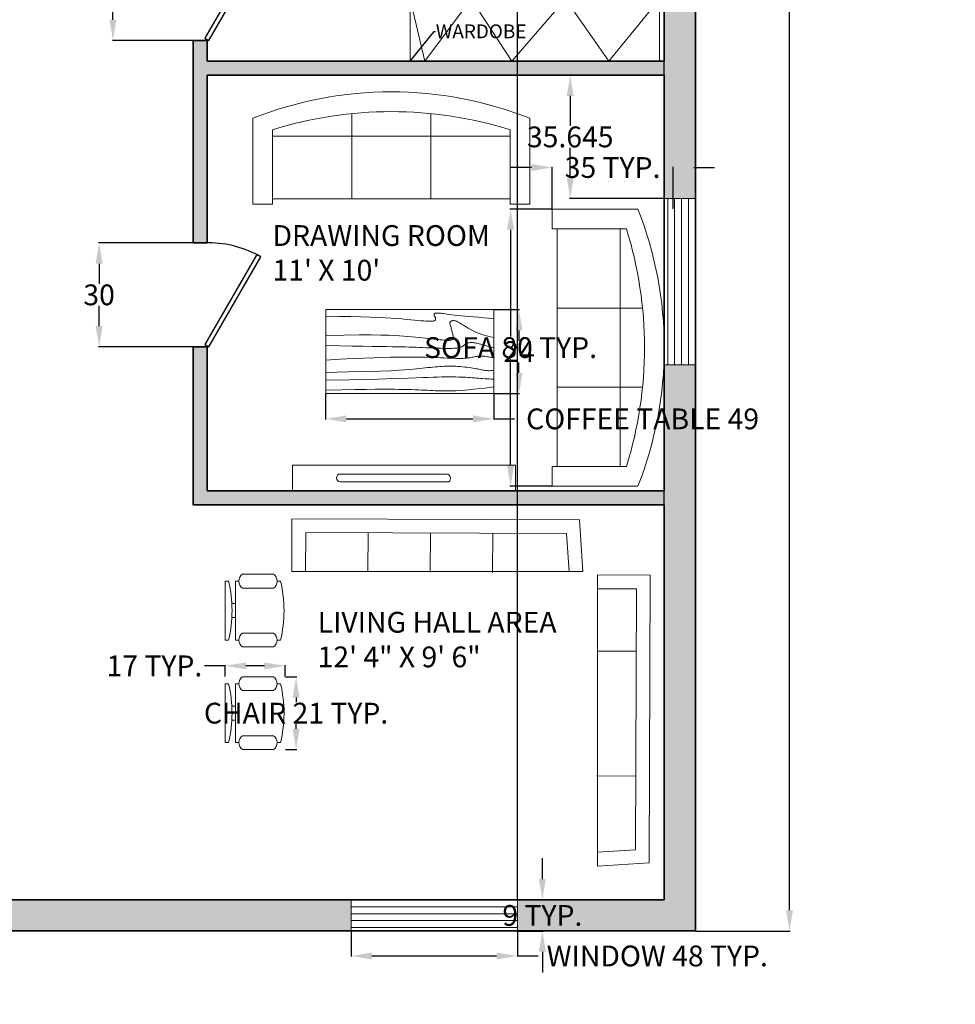
# Model space of a CAD drawing. Units: inches. Extents: x -16 to 578, y -553 to 49.
# Tile 2 of 5: x 308 to 578, y -543 to -259. Entities that reach past the tile are written whole.
import ezdxf
from ezdxf import colors
from ezdxf.entities.mleader import LeaderData, LeaderLine
from ezdxf.math import Vec2, Vec3

# ---------------------------------------------------------------- set-up
doc = ezdxf.new("R2010")
doc.units = ezdxf.units.IN
doc.header["$MEASUREMENT"] = 0
for name, color, linetype, lineweight in [('A-ANNO-DIMS', 2, 'Continuous', 18), ('A-ANNO-TEXT', 7, 'Continuous', 18), ('A-AREA-IDEN', 7, 'Continuous', 25), ('A-DOOR', 3, 'Continuous', 25), ('A-FLOR-CASE', 8, 'Continuous', 18), ('A-FURN', 8, 'Continuous', 18), ('A-GLAZ', 4, 'Continuous', 18), ('A-WALL', 7, 'Continuous', 35)]:
    doc.layers.add(name, color=color, linetype=linetype, lineweight=lineweight)
doc.layers.add('A-WALL-PATT', color=251, linetype='Continuous', lineweight=13, true_color=0x636466)
doc.styles.get("Standard").update_dxf_attribs({"font": 'arial.ttf'})
doc.dimstyles.get("Standard").update_dxf_attribs({"dimtxt": 6, "dimasz": 6, "dimexe": 0.18, "dimexo": 0.0625, "dimgap": 0.09, "dimtad": 0, "dimtih": 1, "dimtoh": 1, "dimdec": 0, "dimzin": 0, "dimdsep": 46, "dimlunit": 4, "dimtxsty": 'Standard', "dimcen": 0.09, "dimadec": 0, "dimazin": 0, "dimtfac": 1, "dimtdec": 0, "dimtofl": 0, "dimtmove": 0, "dimatfit": 3, "dimfxl": 1, "dimtolj": 1, "dimtzin": 0, "dimarcsym": 0})

# ---------------------------------------------------------------- blocks, each defined once
blk = doc.blocks.new('*U4')
for p, q in [((0, 0), (0, -6)), ((-40, 0), (-40, -6))]:
    blk.add_line(p, q)
blk.add_lwpolyline([(0, 0), (-34.64, 20), (-35.52, 18.48), (-0.88, -1.52)], close=True)
blk.add_arc((0, 0), 40, 150, 180)
blk = doc.blocks.new('Chair - Desk')
for p, q in [((-8.5, 0), (-8.5, -1)), ((-8.5, 0), (8.5, 0)), ((8.5, 0), (8.5, -1)), ((-2, -3), (-2, -1.9355)), ((2, -1.9576), (2, -3)), ((-10.5, -5), (-10.5, -14)), ((-8.5, -3), (-8.5, -4)), ((-8.5, -3), (8.5, -3)), ((-6.5, -14), (-6.5, -5)), ((6.5, -5), (6.5, -14)), ((8.5, -3), (8.5, -4)), ((10.5, -14), (10.5, -5)), ((-8.5, -15), (-8.5, -16)), ((8.5, -15), (8.5, -16))]:
    blk.add_line(p, q)
for centre, radius, start, end in [((0, 34.625), 36.625, 256.5803, 283.4197), ((-8.5, -6.5), 2.5, 36.8699, 143.1301), ((8.5, -6.5), 2.5, 36.8699, 143.1301), ((-8.5, -12.5), 2.5, 216.8699, 323.1301), ((8.5, -12.5), 2.5, 216.8699, 323.1301), ((0, 19.625), 36.625, 256.5803, 283.4197)]:
    blk.add_arc(centre, radius, start, end)
blk = doc.blocks.new('Table - Rectangular Woodgrain 60 x 30 in.')
for p, q in [((0, 0), (0, -30)), ((60, 0), (0, 0)), ((60, -30), (60, 0)), ((0, -30), (60, -30))]:
    blk.add_line(p, q)
for points in [[(0, -2.4), (4.8155, -2.418), (9.0302, -2.4688), (12.709, -2.5477), (15.9167, -2.65), (18.7181, -2.7711), (21.1781, -2.9063), (23.3616, -3.0508), (25.3333, -3.2), (27.1477, -3.3495), (28.8172, -3.4958), (30.3437, -3.636), (31.7291, -3.7667), (32.9756, -3.8849), (34.0849, -3.9875), (35.059, -4.0714), (35.9, -4.1334), (36.6114, -4.1711), (37.2041, -4.1854), (37.6906, -4.1779), (38.0833, -4.15), (38.3948, -4.1034), (38.6375, -4.0396), (38.8239, -3.9602), (38.9666, -3.8667), (39.0764, -3.7608), (39.1573, -3.6448), (39.2116, -3.521), (39.2416, -3.3917), (39.2498, -3.2593), (39.2385, -3.1261), (39.21, -2.9944), (39.1666, -2.8667), (39.111, -2.7447), (39.0468, -2.6281), (38.978, -2.5163), (38.9083, -2.4083), (38.8418, -2.3035), (38.7823, -2.201), (38.7337, -2.1001), (38.7, -2), (38.6844, -1.9003), (38.6875, -1.8021), (38.7094, -1.707), (38.75, -1.6167), (38.8094, -1.5326), (38.8875, -1.4563), (38.9844, -1.3893), (39.1, -1.3333), (39.2351, -1.2896), (39.3937, -1.2583), (39.5804, -1.2396), (39.8, -1.2333), (40.057, -1.2396), (40.3562, -1.2583), (40.7023, -1.2896), (41.1, -1.3333), (41.5547, -1.3895), (42.0755, -1.4573), (42.6721, -1.5361), (43.3542, -1.625), (44.1316, -1.7233), (45.014, -1.8302), (46.0114, -1.9449), (47.1333, -2.0667), (48.3862, -2.1947), (49.7625, -2.3281), (51.2513, -2.4663), (52.8416, -2.6083), (54.5226, -2.7535), (56.2833, -2.9011), (58.1127, -3.0501), (60, -3.2)], [(0, -9.2), (6.5759, -9.0858), (11.9385, -9.0365), (16.2527, -9.0418), (19.6833, -9.0917), (22.3952, -9.1759), (24.5531, -9.2844), (26.322, -9.4069), (27.8666, -9.5333), (29.3241, -9.6553), (30.7203, -9.7719), (32.0532, -9.8837), (33.3208, -9.9917), (34.5213, -10.0965), (35.6526, -10.199), (36.7128, -10.2999), (37.7, -10.4), (38.6129, -10.4996), (39.4531, -10.5969), (40.223, -10.6895), (40.925, -10.775), (41.5613, -10.8512), (42.1344, -10.9156), (42.6465, -10.966), (43.1, -11), (43.4976, -11.0158), (43.8437, -11.0136), (44.143, -10.9942), (44.4, -10.9583), (44.6195, -10.9069), (44.8062, -10.8406), (44.9648, -10.7603), (45.1, -10.6667), (45.2155, -10.5598), (45.3114, -10.4365), (45.3871, -10.2929), (45.4416, -10.125), (45.4743, -9.929), (45.4844, -9.7011), (45.4709, -9.4371), (45.4333, -9.1333), (45.3716, -8.7883), (45.2896, -8.4104), (45.1919, -8.0107), (45.0833, -7.6), (44.9685, -7.1893), (44.8521, -6.7896), (44.7388, -6.4117), (44.6333, -6.0667), (44.54, -5.7628), (44.4614, -5.4979), (44.4001, -5.2675), (44.3583, -5.0667), (44.3384, -4.8909), (44.3427, -4.7354), (44.3736, -4.5956), (44.4333, -4.4667), (44.5236, -4.3453), (44.6427, -4.2333), (44.7884, -4.1339), (44.9583, -4.05), (45.1501, -3.9849), (45.3614, -3.9417), (45.59, -3.9234), (45.8333, -3.9333), (46.0915, -3.9749), (46.3734, -4.0531), (46.6906, -4.1736), (47.0542, -4.3417), (47.4756, -4.5629), (47.9661, -4.8427), (48.5372, -5.1866), (49.2, -5.6), (49.9676, -6.0844), (50.8594, -6.625), (51.8965, -7.2031), (53.1, -7.8), (54.491, -8.3969), (56.0906, -8.975), (57.9199, -9.5156), (60, -10)], [(0, -12.8), (5.1847, -12.9322), (9.6213, -13.0323), (13.3963, -13.1059), (16.5958, -13.1583), (19.3063, -13.1952), (21.614, -13.2219), (23.6054, -13.2439), (25.3666, -13.2667), (26.9728, -13.2947), (28.4531, -13.3281), (29.8256, -13.3663), (31.1083, -13.4083), (32.3191, -13.4535), (33.476, -13.501), (34.597, -13.5501), (35.7, -13.6), (36.7984, -13.6497), (37.8875, -13.6979), (38.9578, -13.743), (40, -13.7833), (41.0047, -13.8174), (41.9625, -13.8438), (42.864, -13.8607), (43.7, -13.8667), (44.4631, -13.8604), (45.1552, -13.8417), (45.7801, -13.8104), (46.3416, -13.7667), (46.8439, -13.7104), (47.2906, -13.6417), (47.6858, -13.5604), (48.0333, -13.4667), (48.3375, -13.3608), (48.6042, -13.2448), (48.8396, -13.121), (49.05, -12.9917), (49.2417, -12.8593), (49.4208, -12.7261), (49.5937, -12.5944), (49.7667, -12.4667), (49.9452, -12.3451), (50.1323, -12.2313), (50.3303, -12.1268), (50.5416, -12.0333), (50.7686, -11.9524), (51.0135, -11.8854), (51.2788, -11.8341), (51.5666, -11.8), (51.8785, -11.7843), (52.2116, -11.7865), (52.562, -11.8059), (52.926, -11.8417), (53.2998, -11.8931), (53.6795, -11.9594), (54.0614, -12.0397), (54.4416, -12.1333), (54.8223, -12.2401), (55.2293, -12.3625), (55.6942, -12.5037), (56.2489, -12.6667), (56.9251, -12.8547), (57.7545, -13.0708), (58.7689, -13.3182), (60, -13.6)], [(0, -18), (5.124, -17.7273), (9.6609, -17.5057), (13.6705, -17.3303), (17.2125, -17.1958), (20.3467, -17.0973), (23.1328, -17.0297), (25.6307, -16.9878), (27.9, -16.9667), (29.9928, -16.9617), (31.9302, -16.9703), (33.7254, -16.9907), (35.3917, -17.0208), (36.9423, -17.0588), (38.3906, -17.1026), (39.7499, -17.1503), (41.0333, -17.2), (42.2519, -17.2496), (43.4073, -17.2969), (44.4986, -17.3395), (45.525, -17.375), (46.4858, -17.4012), (47.3802, -17.4156), (48.2074, -17.416), (48.9667, -17.4), (49.6583, -17.3662), (50.2872, -17.3167), (50.8595, -17.2547), (51.3812, -17.1833), (51.8584, -17.1057), (52.2971, -17.025), (52.7034, -16.9443), (53.0833, -16.8667), (53.443, -16.7951), (53.789, -16.7313), (54.128, -16.6768), (54.4666, -16.6334), (54.8115, -16.6024), (55.1693, -16.5854), (55.5465, -16.5841), (55.95, -16.6), (56.3828, -16.6337), (56.8346, -16.6823), (57.2915, -16.7418), (57.7396, -16.8084), (58.165, -16.878), (58.5539, -16.9469), (58.8924, -17.0111), (59.1666, -17.0667), (59.3679, -17.1107), (59.5078, -17.1438), (59.6032, -17.1675), (59.6708, -17.1833), (59.7275, -17.193), (59.7901, -17.1979), (59.8753, -17.1998), (60, -17.2)], [(0, -22.4), (8.0098, -22.2501), (14.4094, -22.1011), (19.4168, -21.9535), (23.25, -21.8083), (26.1269, -21.6663), (28.2656, -21.5281), (29.884, -21.3947), (31.2, -21.2667), (32.3967, -21.1448), (33.5172, -21.0292), (34.5697, -20.9198), (35.5625, -20.8167), (36.5037, -20.7198), (37.4015, -20.6292), (38.2642, -20.5448), (39.1, -20.4667), (39.9164, -20.3951), (40.7187, -20.3313), (41.5117, -20.2768), (42.3, -20.2333), (43.0883, -20.2024), (43.8812, -20.1854), (44.6836, -20.1841), (45.5, -20.2), (46.3328, -20.234), (47.1747, -20.2844), (48.0163, -20.3488), (48.8479, -20.425), (49.66, -20.5106), (50.4429, -20.6031), (51.1872, -20.7004), (51.8833, -20.8), (52.5246, -20.8999), (53.1166, -20.9995), (53.6681, -21.0983), (54.1875, -21.1958), (54.6834, -21.2919), (55.1646, -21.3859), (55.6394, -21.4777), (56.1167, -21.5667), (56.6028, -21.6515), (57.0961, -21.7266), (57.5929, -21.7852), (58.0896, -21.8208), (58.5823, -21.8268), (59.0674, -21.7964), (59.5412, -21.723), (60, -21.6)], [(0, -25.2), (8.6355, -25.0504), (15.7026, -24.9031), (21.4049, -24.7606), (25.9458, -24.625), (29.529, -24.4988), (32.3578, -24.3844), (34.6359, -24.284), (36.5667, -24.2), (38.3213, -24.1341), (39.9417, -24.0854), (41.437, -24.0523), (42.8167, -24.0333), (44.0901, -24.0268), (45.2667, -24.0313), (46.3557, -24.0451), (47.3667, -24.0667), (48.309, -24.0947), (49.1928, -24.1287), (50.0284, -24.168), (50.826, -24.2125), (51.5959, -24.2617), (52.3483, -24.3151), (53.0935, -24.3725), (53.8417, -24.4334), (54.6009, -24.497), (55.3699, -24.561), (56.1454, -24.6226), (56.9239, -24.6792), (57.7021, -24.7279), (58.4764, -24.7662), (59.2435, -24.7911), (60, -24.8)], [(0, -28.8), (5.6867, -28.6681), (10.45, -28.5698), (14.407, -28.5012), (17.675, -28.4584), (20.3711, -28.4374), (22.6125, -28.4344), (24.5164, -28.4455), (26.2, -28.4667), (27.762, -28.4947), (29.2276, -28.5281), (30.6033, -28.5663), (31.8958, -28.6084), (33.1118, -28.6535), (34.2578, -28.7011), (35.3405, -28.7501), (36.3666, -28.8), (37.3443, -28.8497), (38.288, -28.8974), (39.2137, -28.9412), (40.1375, -28.9792), (41.0753, -29.0093), (42.0432, -29.0297), (43.0572, -29.0384), (44.1333, -29.0333), (45.2936, -29.0114), (46.5843, -28.9641), (48.0579, -28.8816), (49.7666, -28.7542), (51.7629, -28.5721), (54.0989, -28.3255), (56.8272, -28.0048), (60, -27.6)]]:
    blk.add_lwpolyline(points)
blk = doc.blocks.new('Sofa - Roundback 7 ft.')
for p, q in [((-12.00002, -32.4421), (-12.00003, -6.5971)), ((11.99997, -32.4421), (11.99998, -6.5971)), ((-36.000027, -34), (-36.000027, -11.4696)), ((35.99998, -34), (35.99998, -11.4696)), ((-35.999844, -13.3819), (35.9998, -13.3819)), ((-36.000027, -32.4421), (35.99998, -32.4421))]:
    blk.add_line(p, q)
for points in [[(-36.000027, -34), (-42.000027, -34), (-42.000027, -8)], [(41.99998, -8), (41.99998, -34), (35.99998, -34)]]:
    blk.add_lwpolyline(points)
for centre, radius, start, end in [((0, -114.25), 114.25, 68.43141, 111.5686), ((-0.00001, -127.1968), 121.1968, 72.72033, 107.2797)]:
    blk.add_arc(centre, radius, start, end)
blk = doc.blocks.new('WIN-48X9')
for p, q in [((-48, -4), (0, -4)), ((-48, -6), (0, -6)), ((-48, -8), (0, -8))]:
    blk.add_line(p, q)
for points in [[(0, 0), (0, -9), (-48, -9), (-48, 0)], [(-48, -2), (0, -2)]]:
    blk.add_lwpolyline(points, close=True)
blk = doc.blocks.new('WARDROBE-72X18')
for p, q in [((0, 0), (18, -14.58)), ((18, -14.58), (0, -27.16)), ((0, -27.16), (18, -42.59)), ((18, -42.59), (0, -54.31)), ((0, -54.31), (18, -67.75)), ((18, -67.75), (0, -72))]:
    blk.add_line(p, q)
blk.add_lwpolyline([(0, 0), (18, 0), (18, -72), (0, -72)], close=True)
blk = doc.blocks.new('*D26')
at = {"layer": 'A-ANNO-DIMS', "color": 0, "lineweight": -2, "transparency": 16777216}
for p, q in [((403.8, -521.83), (403.8, -529.15)), ((451.8, -521.83), (451.8, -529.15)), ((409.8, -528.97), (445.8, -528.97)), ((451.8, -528.97), (457.8, -528.97))]:
    blk.add_line(p, q, dxfattribs=at)
at = {"layer": 'A-ANNO-DIMS', "color": 0, "transparency": 16777216}
for points in [[(409.8, -527.97), (409.8, -529.97), (403.8, -528.97)], [(445.8, -527.97), (445.8, -529.97), (451.8, -528.97)]]:
    blk.add_solid(points, dxfattribs=at)
at = {"layer": 'Defpoints', "color": 0, "transparency": 16777216}
for p in [(403.8, -521.77), (451.8, -521.77), (451.8, -528.97)]:
    blk.add_point(p, dxfattribs=at)
at = {"layer": 'A-ANNO-DIMS', "color": 0, "transparency": 16777216, "insert": (492.17, -528.97), "char_height": 6, "attachment_point": 5}
blk.add_mtext('\\A1;WINDOW 48 TYP.', dxfattribs=at)
blk = doc.blocks.new('*D27')
at = {"layer": 'A-ANNO-DIMS', "color": 0, "lineweight": -2, "transparency": 16777216}
for p, q in [((459, -506.77), (459, -500.77)), ((451.87, -512.77), (459.18, -512.77)), ((451.87, -521.77), (459.18, -521.77)), ((459, -527.77), (459, -533.77))]:
    blk.add_line(p, q, dxfattribs=at)
at = {"layer": 'A-ANNO-DIMS', "color": 0, "transparency": 16777216}
for points in [[(458, -506.77), (460, -506.77), (459, -512.77)], [(458, -527.77), (460, -527.77), (459, -521.77)]]:
    blk.add_solid(points, dxfattribs=at)
at = {"layer": 'Defpoints', "color": 0, "transparency": 16777216}
for p in [(451.8, -512.77), (459, -512.77), (451.8, -521.77)]:
    blk.add_point(p, dxfattribs=at)
at = {"layer": 'A-ANNO-DIMS', "color": 0, "transparency": 16777216, "insert": (459, -517.27), "char_height": 6, "attachment_point": 5}
blk.add_mtext('\\A1;9 TYP.', dxfattribs=at)
blk = doc.blocks.new('*D28')
at = {"layer": 'A-ANNO-DIMS', "color": 0, "lineweight": -2, "transparency": 16777216}
for p, q in [((471.56, -245.54), (471.56, -248.36)), ((489.56, -245.54), (489.56, -248.36)), ((477.56, -248.18), (483.56, -248.18)), ((489.56, -248.18), (495.56, -248.18))]:
    blk.add_line(p, q, dxfattribs=at)
at = {"layer": 'A-ANNO-DIMS', "color": 0, "transparency": 16777216}
for points in [[(477.56, -247.18), (477.56, -249.18), (471.56, -248.18)], [(483.56, -247.18), (483.56, -249.18), (489.56, -248.18)]]:
    blk.add_solid(points, dxfattribs=at)
at = {"layer": 'Defpoints', "color": 0, "transparency": 16777216}
for p in [(471.56, -245.48), (489.56, -245.48), (489.56, -248.18)]:
    blk.add_point(p, dxfattribs=at)
at = {"layer": 'A-ANNO-DIMS', "color": 0, "transparency": 16777216, "insert": (538.51, -248.18), "char_height": 6, "attachment_point": 5}
blk.add_mtext('\\A1;NIGHTSTAND 18 TYP.', dxfattribs=at)
blk = doc.blocks.new('*D36')
at = {"layer": 'A-ANNO-DIMS', "color": 0, "lineweight": -2, "transparency": 16777216}
for p, q in [((384.81, -448.4), (388.08, -448.4)), ((387.9, -454.4), (387.9, -455.71)), ((387.9, -463.4), (387.9, -462.09)), ((384.81, -469.4), (388.08, -469.4))]:
    blk.add_line(p, q, dxfattribs=at)
at = {"layer": 'A-ANNO-DIMS', "color": 0, "transparency": 16777216}
for points in [[(386.9, -454.4), (388.9, -454.4), (387.9, -448.4)], [(386.9, -463.4), (388.9, -463.4), (387.9, -469.4)]]:
    blk.add_solid(points, dxfattribs=at)
at = {"layer": 'Defpoints', "color": 0, "transparency": 16777216}
for p in [(384.75, -448.4), (387.9, -448.4), (384.75, -469.4)]:
    blk.add_point(p, dxfattribs=at)
at = {"layer": 'A-ANNO-DIMS', "color": 0, "transparency": 16777216, "insert": (387.9, -458.9), "char_height": 6, "attachment_point": 5}
blk.add_mtext('\\A1;CHAIR 21 TYP.', dxfattribs=at)
blk = doc.blocks.new('*D37')
at = {"layer": 'A-ANNO-DIMS', "color": 0, "lineweight": -2, "transparency": 16777216}
for p, q in [((367.42, -445.25), (361.42, -445.25)), ((367.42, -448.34), (367.42, -445.07)), ((378.75, -445.25), (373.42, -445.25)), ((384.75, -448.34), (384.75, -445.07))]:
    blk.add_line(p, q, dxfattribs=at)
at = {"layer": 'A-ANNO-DIMS', "color": 0, "transparency": 16777216}
for points in [[(373.42, -444.25), (373.42, -446.25), (367.42, -445.25)], [(378.75, -444.25), (378.75, -446.25), (384.75, -445.25)]]:
    blk.add_solid(points, dxfattribs=at)
at = {"layer": 'Defpoints', "color": 0, "transparency": 16777216}
for p in [(367.42, -445.25), (367.42, -448.4), (384.75, -448.4)]:
    blk.add_point(p, dxfattribs=at)
at = {"layer": 'A-ANNO-DIMS', "color": 0, "transparency": 16777216, "insert": (347.01, -445.25), "char_height": 6, "attachment_point": 5}
blk.add_mtext('\\A1;17 TYP.', dxfattribs=at)
blk = doc.blocks.new('*D42')
at = {"layer": 'A-ANNO-DIMS', "color": 0, "lineweight": -2, "transparency": 16777216}
for p, q in [((461.75, -313.41), (449.64, -313.41)), ((449.82, -319.41), (449.82, -350.21)), ((449.82, -387.39), (449.82, -356.6)), ((461.75, -393.39), (449.64, -393.39))]:
    blk.add_line(p, q, dxfattribs=at)
at = {"layer": 'A-ANNO-DIMS', "color": 0, "transparency": 16777216}
for points in [[(448.82, -319.41), (450.82, -319.41), (449.82, -313.41)], [(448.82, -387.39), (450.82, -387.39), (449.82, -393.39)]]:
    blk.add_solid(points, dxfattribs=at)
at = {"layer": 'Defpoints', "color": 0, "transparency": 16777216}
for p in [(449.82, -313.41), (461.82, -313.41), (461.82, -393.39)]:
    blk.add_point(p, dxfattribs=at)
at = {"layer": 'A-ANNO-DIMS', "color": 0, "transparency": 16777216, "insert": (449.82, -353.4), "char_height": 6, "attachment_point": 5}
blk.add_mtext('\\A1;SOFA 80 TYP.', dxfattribs=at)
blk = doc.blocks.new('*D43')
at = {"layer": 'A-ANNO-DIMS', "color": 0, "lineweight": -2, "transparency": 16777216}
for p, q in [((455.82, -301.42), (449.82, -301.42)), ((461.82, -313.35), (461.82, -301.24)), ((496.73, -313.35), (496.73, -301.24)), ((502.73, -301.42), (508.73, -301.42))]:
    blk.add_line(p, q, dxfattribs=at)
at = {"layer": 'A-ANNO-DIMS', "color": 0, "transparency": 16777216}
for points in [[(455.82, -300.42), (455.82, -302.42), (461.82, -301.42)], [(502.73, -300.42), (502.73, -302.42), (496.73, -301.42)]]:
    blk.add_solid(points, dxfattribs=at)
at = {"layer": 'Defpoints', "color": 0, "transparency": 16777216}
for p in [(496.73, -301.42), (461.82, -313.41), (496.73, -313.41)]:
    blk.add_point(p, dxfattribs=at)
at = {"layer": 'A-ANNO-DIMS', "color": 0, "transparency": 16777216, "insert": (479.27, -301.42), "char_height": 6, "attachment_point": 5}
blk.add_mtext('\\A1;35 TYP.', dxfattribs=at)
blk = doc.blocks.new('*D58')
at = {"layer": 'A-ANNO-DIMS', "color": 0, "lineweight": -2, "transparency": 16777216}
for p, q in [((396.44, -366.75), (396.44, -374.15)), ((444.97, -366.75), (444.97, -374.15)), ((402.44, -373.97), (438.97, -373.97)), ((444.97, -373.97), (450.97, -373.97))]:
    blk.add_line(p, q, dxfattribs=at)
at = {"layer": 'A-ANNO-DIMS', "color": 0, "transparency": 16777216}
for points in [[(402.44, -372.97), (402.44, -374.97), (396.44, -373.97)], [(438.97, -372.97), (438.97, -374.97), (444.97, -373.97)]]:
    blk.add_solid(points, dxfattribs=at)
at = {"layer": 'Defpoints', "color": 0, "transparency": 16777216}
for p in [(396.44, -366.69), (444.97, -366.69), (444.97, -373.97)]:
    blk.add_point(p, dxfattribs=at)
at = {"layer": 'A-ANNO-DIMS', "color": 0, "transparency": 16777216, "insert": (487.93, -373.97), "char_height": 6, "attachment_point": 5}
blk.add_mtext('\\A1;COFFEE TABLE 49', dxfattribs=at)
blk = doc.blocks.new('*D59')
at = {"layer": 'A-ANNO-DIMS', "color": 0, "lineweight": -2, "transparency": 16777216}
for p, q in [((445.03, -342.43), (452.43, -342.43)), ((452.25, -348.43), (452.25, -351.46)), ((452.25, -360.69), (452.25, -357.66)), ((445.03, -366.69), (452.43, -366.69))]:
    blk.add_line(p, q, dxfattribs=at)
at = {"layer": 'A-ANNO-DIMS', "color": 0, "transparency": 16777216}
for points in [[(451.25, -348.43), (453.25, -348.43), (452.25, -342.43)], [(451.25, -360.69), (453.25, -360.69), (452.25, -366.69)]]:
    blk.add_solid(points, dxfattribs=at)
at = {"layer": 'Defpoints', "color": 0, "transparency": 16777216}
for p in [(444.97, -342.43), (452.25, -342.43), (444.97, -366.69)]:
    blk.add_point(p, dxfattribs=at)
at = {"layer": 'A-ANNO-DIMS', "color": 0, "transparency": 16777216, "insert": (452.25, -354.56), "char_height": 6, "attachment_point": 5}
blk.add_mtext('\\A1;24', dxfattribs=at)
blk = doc.blocks.new('*D63')
at = {"layer": 'A-ANNO-DIMS', "color": 0, "lineweight": -2, "transparency": 16777216}
for p, q in [((503.25, 18.23), (530.52, 18.23)), ((530.34, 12.23), (530.34, -248.61)), ((530.34, -515.77), (530.34, -254.92)), ((503.25, -521.77), (530.52, -521.77))]:
    blk.add_line(p, q, dxfattribs=at)
at = {"layer": 'A-ANNO-DIMS', "color": 0, "transparency": 16777216}
for points in [[(529.34, 12.23), (531.34, 12.23), (530.34, 18.23)], [(529.34, -515.77), (531.34, -515.77), (530.34, -521.77)]]:
    blk.add_solid(points, dxfattribs=at)
at = {"layer": 'Defpoints', "color": 0, "transparency": 16777216}
for p in [(503.19, 18.23), (503.19, -521.77), (530.34, -521.77)]:
    blk.add_point(p, dxfattribs=at)
at = {"layer": 'A-ANNO-DIMS', "color": 0, "transparency": 16777216, "insert": (530.34, -251.77), "char_height": 6, "attachment_point": 5}
blk.add_mtext('\\A1;540', dxfattribs=at)
blk = doc.blocks.new('*D70')
at = {"layer": 'A-ANNO-DIMS', "color": 0, "lineweight": -2, "transparency": 16777216}
for p, q in [((362.13, -234.77), (334.86, -234.77)), ((335.04, -240.77), (335.04, -246.61)), ((335.04, -258.77), (335.04, -252.92)), ((362.13, -264.77), (334.86, -264.77))]:
    blk.add_line(p, q, dxfattribs=at)
at = {"layer": 'A-ANNO-DIMS', "color": 0, "transparency": 16777216}
for points in [[(334.04, -240.77), (336.04, -240.77), (335.04, -234.77)], [(334.04, -258.77), (336.04, -258.77), (335.04, -264.77)]]:
    blk.add_solid(points, dxfattribs=at)
at = {"layer": 'Defpoints', "color": 0, "transparency": 16777216}
for p in [(335.04, -234.77), (362.19, -234.77), (362.19, -264.77)]:
    blk.add_point(p, dxfattribs=at)
at = {"layer": 'A-ANNO-DIMS', "color": 0, "transparency": 16777216, "insert": (335.04, -249.77), "char_height": 6, "attachment_point": 5}
blk.add_mtext('\\A1;30', dxfattribs=at)
blk = doc.blocks.new('*D77')
at = {"layer": 'A-ANNO-DIMS', "color": 0, "lineweight": -2, "transparency": 16777216}
for p, q in [((494.13, -274.77), (466.86, -274.77)), ((467.04, -280.77), (467.04, -289.43)), ((467.04, -304.41), (467.04, -295.74)), ((494.13, -310.41), (466.86, -310.41))]:
    blk.add_line(p, q, dxfattribs=at)
at = {"layer": 'A-ANNO-DIMS', "color": 0, "transparency": 16777216}
for points in [[(466.04, -280.77), (468.04, -280.77), (467.04, -274.77)], [(466.04, -304.41), (468.04, -304.41), (467.04, -310.41)]]:
    blk.add_solid(points, dxfattribs=at)
at = {"layer": 'Defpoints', "color": 0, "transparency": 16777216}
for p in [(467.04, -274.77), (494.19, -274.77), (494.19, -310.41)]:
    blk.add_point(p, dxfattribs=at)
at = {"layer": 'A-ANNO-DIMS', "color": 0, "transparency": 16777216, "insert": (467.04, -292.59), "char_height": 6, "attachment_point": 5}
blk.add_mtext('\\A1;35.645', dxfattribs=at)
blk = doc.blocks.new('*D80')
at = {"layer": 'A-ANNO-DIMS', "color": 0, "lineweight": -2, "transparency": 16777216}
for p, q in [((451.8, -512.7), (451.8, 45.56)), ((494.19, -512.7), (494.19, 45.56)), ((457.8, 45.38), (462.66, 45.38)), ((488.19, 45.38), (483.34, 45.38))]:
    blk.add_line(p, q, dxfattribs=at)
at = {"layer": 'A-ANNO-DIMS', "color": 0, "transparency": 16777216}
for points in [[(457.8, 46.38), (457.8, 44.38), (451.8, 45.38)], [(488.19, 46.38), (488.19, 44.38), (494.19, 45.38)]]:
    blk.add_solid(points, dxfattribs=at)
at = {"layer": 'Defpoints', "color": 0, "transparency": 16777216}
for p in [(451.8, 45.38), (451.8, -512.77), (494.19, -512.77)]:
    blk.add_point(p, dxfattribs=at)
at = {"layer": 'A-ANNO-DIMS', "color": 0, "transparency": 16777216, "insert": (473, 45.38), "char_height": 6, "attachment_point": 5}
blk.add_mtext('\\A1;42.38', dxfattribs=at)
blk = doc.blocks.new('*D85')
at = {"layer": 'A-ANNO-DIMS', "color": 0, "lineweight": -2, "transparency": 16777216}
for p, q in [((358.13, -323.18), (330.86, -323.18)), ((331.04, -329.18), (331.04, -335.02)), ((331.04, -347.18), (331.04, -341.33)), ((358.13, -353.18), (330.86, -353.18))]:
    blk.add_line(p, q, dxfattribs=at)
at = {"layer": 'A-ANNO-DIMS', "color": 0, "transparency": 16777216}
for points in [[(330.04, -329.18), (332.04, -329.18), (331.04, -323.18)], [(330.04, -347.18), (332.04, -347.18), (331.04, -353.18)]]:
    blk.add_solid(points, dxfattribs=at)
at = {"layer": 'Defpoints', "color": 0, "transparency": 16777216}
for p in [(331.04, -323.18), (358.19, -323.18), (358.19, -353.18)]:
    blk.add_point(p, dxfattribs=at)
at = {"layer": 'A-ANNO-DIMS', "color": 0, "transparency": 16777216, "insert": (331.04, -338.18), "char_height": 6, "attachment_point": 5}
blk.add_mtext('\\A1;30', dxfattribs=at)

msp = doc.modelspace()

# ---------------------------------------------------------------- hatches: boundary and pattern name
at = {"layer": 'A-WALL-PATT'}
h = msp.add_hatch(color=256, dxfattribs=at)
h.dxf.hatch_style = 1
h.paths.add_polyline_path([(32.1882, 9.2337), (89.8211, 9.2337), (89.8211, 18.2337), (23.1882, 18.2337), (23.1882, -55.5259), (32.1882, -55.5259)])
h.paths.add_polyline_path([(219.6411, 18.2337), (137.8211, 18.2337), (137.8211, 9.2337), (146.4179, 9.2337), (188.1882, 9.2337), (188.1882, -98.7663), (192.1882, -98.7663), (192.1882, -72.7663), (238.1882, -72.7663), (238.1882, -68.7663), (192.1882, -68.7663), (192.1882, 9.2337), (219.6411, 9.2337)])
h.paths.add_polyline_path([(307.3924, 18.2337), (243.6411, 18.2337), (243.6411, 9.2337), (274.1882, 9.2337), (274.1882, -26.7663), (274.1882, -68.7663), (268.1882, -68.7663), (268.1882, -72.7663), (274.1882, -72.7663), (274.1882, -98.7663), (250.1882, -98.7663), (250.1882, -102.7663), (274.1882, -102.7663), (278.1882, -102.7663), (302.188, -102.8481), (302.188, -98.8481), (278.1882, -98.7663), (278.1882, -86.8559, -0.01827889), (278.1882, -85.7663), (278.1882, -72.7663), (284.1882, -72.7663), (284.1882, -68.7663), (278.1882, -68.7663), (278.1882, 9.2337), (307.3924, 9.2337)])
h.paths.add_polyline_path([(402.6701, 18.2337), (331.3924, 18.2337), (331.3924, 9.2337), (358.1882, 9.2337), (358.1882, -26.7663), (358.1882, -68.7663), (314.1882, -68.7663), (314.1882, -72.7663), (358.1882, -72.7663), (358.1882, -98.7663), (362.1882, -98.7663), (362.1882, 9.2337), (402.6701, 9.2337)])
h.paths.add_polyline_path([(503.1882, 18.2337), (450.6701, 18.2337), (450.6701, 9.2337), (462.8072, 9.2337), (494.1882, 9.2337), (494.1882, -38.053), (503.1882, -38.053)])
h.paths.add_polyline_path([(503.1882, -86.053), (494.1882, -86.053), (494.1882, -134.7663), (362.1882, -134.7663), (362.1882, -128.7663), (358.1882, -128.7663), (358.1882, -138.7663), (358.1882, -234.7663), (362.1882, -234.7663), (362.1882, -138.7663), (494.1882, -138.7663), (494.1882, -181.1501), (503.1882, -181.1501)])
h.paths.add_polyline_path([(503.1882, -229.1501), (494.1882, -229.1501), (494.1882, -270.7663), (362.1882, -270.7663), (362.1882, -264.7663), (358.1882, -264.7663), (358.1882, -294.7663), (358.1882, -323.1753), (362.1882, -323.1753), (362.1882, -298.7663), (362.1882, -294.7663), (362.1882, -274.7663), (494.1882, -274.7663), (494.1882, -294.7663), (494.1882, -298.7663), (494.1882, -310.411), (503.1882, -310.411)])
h.paths.add_polyline_path([(503.1882, -358.411), (494.1882, -358.411), (494.1882, -394.7663), (362.1882, -394.7663), (362.1882, -353.1753), (358.1882, -353.1753), (358.1882, -398.7663), (494.1882, -398.7663), (494.1882, -512.7663), (451.8049, -512.7663), (451.8049, -521.7663), (503.1882, -521.7663)])
h.paths.add_polyline_path([(403.8049, -512.7663), (176.1882, -512.7663), (176.1882, -441.7663), (172.1882, -441.7663), (172.1882, -512.7663), (150.1882, -512.7663), (150.1882, -521.7663), (403.8049, -521.7663)])
h.paths.add_polyline_path([(176.1882, -258.7663), (168.1882, -258.7663), (168.1882, -246.7663), (168.1882, -234.7663), (168.1882, -222.7663), (164.1882, -222.7663), (164.1882, -234.7663), (164.1882, -258.7663), (102.0641, -258.7663), (102.0641, -262.7663), (168.1882, -262.7663), (172.1882, -262.7663), (172.1882, -333.7663), (176.1882, -333.7663), (176.1882, -262.7663)])
h.paths.add_polyline_path([(32.1882, -262.7663), (54.0641, -262.7663), (54.0641, -258.7663), (32.1882, -258.7663), (32.1882, -229.1501), (23.1882, -229.1501), (23.1882, -283.4909), (23.1882, -470.2771), (32.1882, -470.2771), (32.1882, -283.4909)])
h.paths.add_polyline_path([(32.1882, -103.5259), (23.1882, -103.5259), (23.1882, -181.1501), (32.1882, -181.1501)])
h.paths.add_polyline_path([(192.1882, -128.7663), (188.1882, -128.7663), (188.1882, -134.7663), (32.1882, -134.7663), (32.1882, -138.7663), (164.1882, -138.7663), (164.1882, -162.7663), (164.1882, -174.7663), (168.1882, -174.7663), (168.1882, -162.7663), (168.1882, -138.7663), (192.1882, -138.7663)])

# ---------------------------------------------------------------- linework, layer by layer
at = {"layer": 'A-FURN'}
for p, q in [((428.5118, -398.7259), (439.7872, -398.7673)), ((386.6271, -418.047), (386.6832, -402.7716)), ((386.6832, -402.7716), (469.7558, -403.0767)), ((469.7558, -403.0767), (470.6981, -418.047)), ((390.6271, -418.0617), (390.6685, -406.7862)), ((390.6685, -406.7862), (465.9988, -407.0629)), ((408.627, -418.1278), (408.6684, -406.8523)), ((426.6269, -418.1939), (426.6683, -406.9184)), ((444.6267, -418.26), (444.6682, -406.9846)), ((465.9988, -407.0629), (466.6902, -418.047)), ((470.6981, -418.047), (386.6271, -418.047)), ((474.8721, -503.0711), (474.8721, -419.0001)), ((474.8721, -419.0001), (490.1476, -419.0562)), ((490.1476, -419.0562), (489.8425, -502.1288)), ((474.8574, -423.0001), (486.1329, -423.0415)), ((486.1329, -423.0415), (485.8562, -498.3718)), ((474.7913, -440.9999), (486.0668, -441.0413)), ((474.6591, -476.9997), (485.9346, -477.0411)), ((485.8562, -498.3718), (474.8721, -499.0632)), ((489.8425, -502.1288), (474.8721, -503.0711))]:
    msp.add_line(p, q, dxfattribs=at)
msp.add_lwpolyline([(386.8421, -387.2836), (451.2251, -387.2836), (451.2251, -394.7663), (386.8421, -394.7663)], close=True, dxfattribs=at)
for points in [[(400.6592, -389.882), (431.5778, -389.882)], [(432.0165, -392.1028), (400.6592, -392.1028)]]:
    msp.add_lwpolyline(points, dxfattribs=at)
for centre, radius, start, end in [((400.6592, -390.9924), 1.1104, 90, 270), ((431.1414, -391.122), 1.3145, 311.737395, 70.613978)]:
    msp.add_arc(centre, radius, start, end, dxfattribs=at)
at = {"layer": 'A-WALL'}
for p, q in [((494.1882, -138.7663), (494.1882, -270.7663)), ((362.1882, -264.7663), (358.1882, -264.7663)), ((358.1882, -264.7663), (358.1882, -294.7663)), ((362.1882, -264.7663), (362.1882, -270.7663)), ((358.1882, -270.7663), (358.1882, -274.7663)), ((362.1882, -270.7663), (494.1882, -270.7663)), ((362.1882, -274.7663), (494.1882, -274.7663)), ((362.1882, -274.7663), (362.1882, -294.7663)), ((494.1882, -274.7663), (494.1882, -294.7663)), ((358.1882, -294.7663), (358.1882, -323.1753)), ((362.1882, -294.7663), (362.1882, -298.7663)), ((494.1882, -294.7663), (494.1882, -298.7663)), ((362.1882, -298.7663), (362.1882, -323.1753)), ((494.1882, -298.7663), (494.1882, -394.7663)), ((362.1882, -323.1753), (358.1882, -323.1753)), ((362.1882, -353.1753), (358.1882, -353.1753)), ((358.1882, -353.1753), (358.1882, -398.7663)), ((362.1882, -353.1753), (362.1882, -394.7663)), ((362.1882, -394.7663), (494.1882, -394.7663)), ((358.1882, -398.7663), (494.1882, -398.7663)), ((494.1882, -398.7663), (494.1882, -512.7663)), ((494.1882, -512.7663), (176.1882, -512.7663)), ((358.1882, -512.7663), (176.1882, -512.7663))]:
    msp.add_line(p, q, dxfattribs=at)
msp.add_lwpolyline([(23.1882, -283.4909), (23.1882, 18.2337), (503.1882, 18.2337), (503.1882, -521.7663), (150.1882, -521.7663)], dxfattribs=at)

# ---------------------------------------------------------------- block references
at = {"layer": 'A-DOOR', "xscale": 0.75, "yscale": 0.75, "zscale": 0.75, "rotation": 270}
for p in [(362.6882, -264.7663), (362.6882, -353.1753)]:
    msp.add_blockref('*U4', p, dxfattribs=at)
at = {"layer": 'A-FLOR-CASE', "rotation": 270.0000000000002}
msp.add_blockref('WARDROBE-72X18', (492.8002, -252.7663), dxfattribs=at)
at = {"layer": 'A-FURN'}
for name, p, xscale, yscale, zscale in [('Sofa - Roundback 7 ft.', (415.3805, -279.5946), 0.9520939681655031, 0.9520939681655031, 0.9520939681655031), ('Table - Rectangular Woodgrain 60 x 30 in.', (396.4415, -342.4272), 0.808763507160089, 0.808763507160089, 0.808763507160089)]:
    msp.add_blockref(name, p, dxfattribs=dict(at, xscale=xscale, yscale=yscale, zscale=zscale))
at = {"layer": 'A-FURN', "xscale": -0.9520939681655031, "yscale": 0.9520939681655031, "zscale": 0.9520939681655031, "rotation": 270}
msp.add_blockref('Sofa - Roundback 7 ft.', (494.1882, -353.4018), dxfattribs=at)
at = {"layer": 'A-FURN', "rotation": 90}
for p in [(367.4171, -429.2976), (367.4171, -458.9019)]:
    msp.add_blockref('Chair - Desk', p, dxfattribs=at)
at = {"layer": 'A-GLAZ', "rotation": 270.0000000000002}
msp.add_blockref('WIN-48X9', (503.1882, -358.411), dxfattribs=at)
at = {"layer": 'A-GLAZ'}
msp.add_blockref('WIN-48X9', (451.8049, -512.7663), dxfattribs=at)

# ---------------------------------------------------------------- texts
at = {"layer": 'A-AREA-IDEN', "char_height": 6, "attachment_point": 1}
for s, width, insert in [("DRAWING ROOM \\P11' X 10'", 70.127107, (381.098, -318.0627)), ('LIVING HALL AREA\\P12\' 4" X 9\' 6"', 95.864796, (394.1302, -429.6612))]:
    msp.add_mtext_dynamic_manual_height_columns(s, width=width, gutter_width=1, heights=[0], dxfattribs=dict(at, insert=insert))

# ---------------------------------------------------------------- dimensions: what is measured, and where the dimension line sits
at = {"layer": 'A-ANNO-DIMS'}
dim = msp.add_linear_dim(base=(451.8049, 45.3837), p1=(494.1882, -512.7663), p2=(451.8049, -512.7663), dimstyle='Standard', override={"dimdec": 2, "dimlfac": 1, "dimrnd": 0, "dimzin": 0, "dimdsep": 46, "dimlunit": 2}, dxfattribs=at)
dim.commit()
dim.dimension.update_dxf_attribs({"geometry": '*D80', "text_midpoint": (472.9965, 45.3837)})
for base, p1, p2, override, picture, middle in [((530.3382, -521.7663), (503.1882, 18.2337), (503.1882, -521.7663), {"dimdec": 0, "dimlfac": 1, "dimrnd": 0, "dimzin": 0, "dimdsep": 46, "dimlunit": 2}, '*D63', (530.3382, -251.7663)), ((335.0382, -234.7663), (362.1882, -264.7663), (362.1882, -234.7663), {"dimdec": 0, "dimlfac": 1, "dimrnd": 0, "dimzin": 0, "dimdsep": 46, "dimlunit": 2}, '*D70', (335.0382, -249.7663)), ((467.0382, -274.7663), (494.1882, -310.411), (494.1882, -274.7663), {"dimdec": 3, "dimlfac": 1, "dimrnd": 0, "dimzin": 0, "dimdsep": 46, "dimlunit": 2}, '*D77', (467.0382, -292.5886)), ((331.0382, -323.1753), (358.1882, -353.1753), (358.1882, -323.1753), {"dimdec": 0, "dimlfac": 1, "dimrnd": 0, "dimzin": 0, "dimdsep": 46, "dimlunit": 2}, '*D85', (331.0382, -338.1753)), ((452.2461, -342.4272), (444.9673, -366.6901), (444.9673, -342.4272), {"dimdec": 0, "dimlfac": 1, "dimrnd": 0, "dimzin": 0, "dimdsep": 46, "dimlunit": 2}, '*D59', (452.2461, -354.5587))]:
    dim = msp.add_linear_dim(base=base, p1=p1, p2=p2, angle=90, dimstyle='Standard', override=override, dxfattribs=at)
    dim.commit()
    dim.dimension.update_dxf_attribs({"geometry": picture, "text_midpoint": middle})
for base, p1, p2, text, picture, middle in [((489.5554, -248.1807), (471.5554, -245.4807), (489.5554, -245.4807), 'NIGHTSTAND <> TYP.', '*D28', (538.509, -248.1807)), ((496.7271, -301.4174), (461.817, -313.4138), (496.7271, -313.4138), '<> TYP.', '*D43', (479.272, -301.4174)), ((444.9673, -373.969), (396.4415, -366.6901), (444.9673, -366.6901), 'COFFEE TABLE <>', '*D58', (487.929, -373.969)), ((451.8049, -528.9663), (403.8049, -521.7663), (451.8049, -521.7663), 'WINDOW <> TYP.', '*D26', (492.1739, -528.9663))]:
    dim = msp.add_linear_dim(base=base, p1=p1, p2=p2, text=text, dimstyle='Standard', override={"dimdec": 0, "dimlfac": 1, "dimrnd": 0, "dimzin": 0, "dimdsep": 46, "dimlunit": 2}, dxfattribs=at)
    dim.commit()
    dim.dimension.update_dxf_attribs({"geometry": picture, "text_midpoint": middle})
for base, p1, p2, angle, text, picture, middle in [((449.8206, -313.4138), (461.817, -393.3897), (461.817, -313.4138), 90, 'SOFA <> TYP.', '*D42', (449.8206, -353.4018)), ((367.4171, -445.2519), (384.7504, -448.4019), (367.4171, -448.4019), 180, '<> TYP.', '*D37', (347.0065, -445.2519)), ((387.9004, -448.4019), (384.7504, -469.4019), (384.7504, -448.4019), 90, 'CHAIR <> TYP.', '*D36', (387.9004, -458.9019)), ((459.0049, -512.7663), (451.8049, -521.7663), (451.8049, -512.7663), 90, '<> TYP.', '*D27', (459.0049, -517.2663))]:
    dim = msp.add_linear_dim(base=base, p1=p1, p2=p2, angle=angle, text=text, dimstyle='Standard', override={"dimdec": 0, "dimlfac": 1, "dimrnd": 0, "dimzin": 0, "dimdsep": 46, "dimlunit": 2}, dxfattribs=at)
    dim.commit()
    dim.dimension.update_dxf_attribs({"geometry": picture, "text_midpoint": middle})

# ---------------------------------------------------------------- leaders
at = {"layer": 'A-ANNO-TEXT'}
ml = msp.add_multileader_mtext('Standard', dxfattribs=at)
ml.set_content('WARDOBE', color=256)
ml.set_leader_properties()
ml.build(insert=Vec2(0, 0))
ml.multileader.update_dxf_attribs({"dogleg_length": 0.36, "arrow_head_size": 0})
ctx = ml.context
ctx.base_point, ctx.arrow_head_size, ctx.landing_gap_size, ctx.plane_origin = Vec3(428.1314, -262.1589), 0, 0.09, Vec3(420.8002, -270.7663)
notes = []
notes.append((ctx, [(0, (1, 1, 0), (427.7714, -262.1589), (1, 0), 0.36, [(0, [(420.8002, -270.7663)], 0, [])])]))
ctx.mtext.insert, ctx.mtext.width, ctx.mtext.flow_direction = Vec3(428.2214, -260.1248), 4, 5
for ctx, leaders in notes:
    for number, flags, end, landing, length, lines in leaders:
        leader = LeaderData()
        leader.index, (leader.has_last_leader_line, leader.has_dogleg_vector, leader.attachment_direction) = number, flags
        leader.last_leader_point, leader.dogleg_vector, leader.dogleg_length = Vec3(end), Vec3(landing), length
        for number, points, colour, breaks in lines:
            line = LeaderLine()
            line.index, line.vertices, line.color, line.breaks = number, Vec3.list(points), colors.encode_raw_color(colour), breaks
            leader.lines.append(line)
        ctx.leaders.append(leader)

doc.saveas('drawing.dxf')
